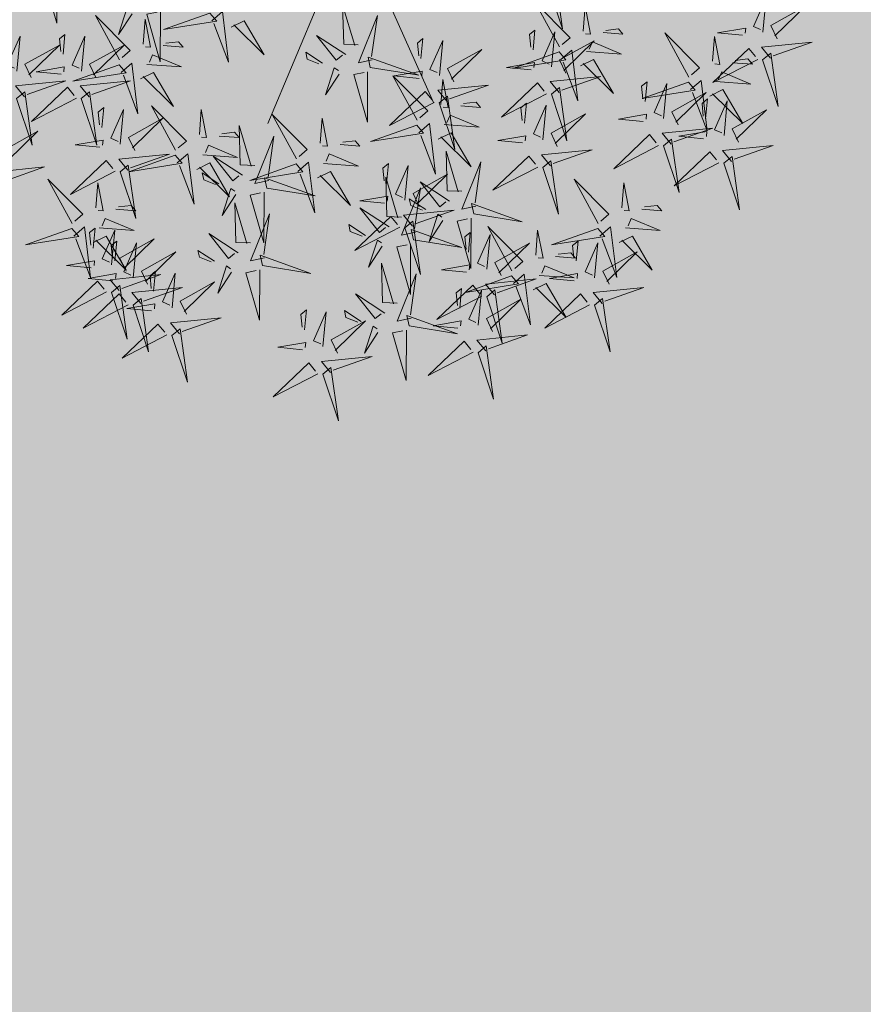
# Model space of a CAD drawing. Units: inches. Extents: x 1704 to 6393, y -157 to 1172.
# Tile 69 of 122: x 1928 to 1954, y 980 to 1010. Entities that reach past the tile are written whole.
import ezdxf

# ---------------------------------------------------------------- set-up
doc = ezdxf.new("R2010")
doc.units = ezdxf.units.IN
doc.header["$MEASUREMENT"] = 0
for name, color, linetype, lineweight in [('A-ANNO-DIMS', 7, 'Continuous', 13), ('L-shrub', 74, 'Continuous', 18), ('L-tree', 102, 'Continuous', 18)]:
    doc.layers.add(name, color=color, linetype=linetype, lineweight=lineweight)
doc.layers.add('L-HRDS-PATT', color=9, linetype='Continuous', lineweight=13, true_color=0xc5c1ba)
doc.styles.get("Standard").update_dxf_attribs({"font": 'arial.ttf'})
doc.dimstyles.get("Standard").update_dxf_attribs({"dimtxt": 6, "dimasz": 2, "dimexe": 0.18, "dimexo": 0.0625, "dimgap": 0.09, "dimtad": 0, "dimtih": 1, "dimtoh": 1, "dimdec": 1, "dimzin": 0, "dimdsep": 46, "dimlunit": 3, "dimtxsty": 'Standard', "dimblk": 'ARCHTICK', "dimcen": 0.09, "dimadec": 0, "dimazin": 0, "dimtfac": 1, "dimtdec": 1, "dimtofl": 0, "dimtmove": 0, "dimatfit": 3, "dimfxl": 1, "dimtolj": 1, "dimtzin": 0, "dimarcsym": 0})

# ---------------------------------------------------------------- blocks, each defined once
blk = doc.blocks.new('bamboo')
at = {"layer": 'L-shrub'}
for p, q in [((43.5, 73), (278.2, 631.2)), ((-12.4, 39.5), (-247.1, 564.2))]:
    blk.add_line(p, q, dxfattribs=at)
for points in [[(103.7, 1424.7), (54.4, 1572.3), (77.9, 1403.4), (103.7, 1424.7)], [(-387.8, 1356.5), (-437.1, 1504.1), (-413.6, 1335.2), (-387.8, 1356.5)], [(119.4, 1423.2), (261.4, 1496.7), (147.9, 1388.7), (126.6, 1414.5)], [(-160.7, 1284.9), (-160, 1444.8), (-116.9, 1294.1), (-149.7, 1287.2)], [(581.6, 1302), (532.2, 1449.6), (555.7, 1280.7), (581.6, 1302)], [(-372, 1355), (-230.1, 1428.5), (-343.6, 1320.5), (-364.9, 1346.4)], [(79.4, 1419.1), (107.8, 1384.6), (-52.4, 1368.4), (70.8, 1412)], [(597.3, 1300.4), (739.2, 1374), (625.7, 1265.9), (604.4, 1291.8)], [(-756.4, 1206.5), (-805.8, 1354.1), (-782.2, 1185.2), (-756.4, 1206.5)], [(-412.1, 1350.9), (-383.7, 1316.4), (-543.9, 1300.2), (-420.7, 1343.8)], [(-70.9, 1292.4), (-27.7, 1358.5), (-55.4, 1272.9), (-68.6, 1281.5)], [(57.7, 1357.7), (77.5, 1316.1), (-31.5, 1255.3), (64.8, 1349.1)], [(167.7, 1347.1), (246.3, 1339.5), (157.6, 1324.2), (159.1, 1340)], [(704.4, 1206.5), (655.1, 1354.1), (678.6, 1185.2), (704.4, 1206.5)], [(-415.1, 1179.2), (-464.4, 1326.8), (-440.9, 1157.9), (-415.1, 1179.2)], [(103.3, 1337.4), (92.8, 1227.4), (133.3, 1318.7), (110.4, 1328.8)], [(772.7, 1165.6), (723.3, 1313.2), (746.9, 1144.3), (772.7, 1165.6)], [(-740.7, 1205), (-598.8, 1278.5), (-712.2, 1170.5), (-733.6, 1196.4)], [(-433.8, 1289.5), (-414, 1248), (-523, 1187.1), (-426.7, 1280.9)], [(-323.8, 1278.9), (-245.2, 1271.3), (-333.9, 1256.1), (-332.4, 1271.8)], [(-169.3, 1271.7), (-323, 1296.4), (-162.4, 1238.9), (-169.3, 1271.7)], [(161.7, 1284.2), (155.7, 1221.3), (172.9, 1235.5), (168.8, 1275.6)], [(557.2, 1296.4), (585.7, 1261.9), (425.4, 1245.7), (548.6, 1289.3)], [(720.2, 1205), (862.1, 1278.5), (748.6, 1170.5), (727.3, 1196.4)], [(-500.1, 1137.3), (-534, 1108.2), (-553.5, 1268), (-507.4, 1145.8)], [(-399.4, 1177.7), (-257.4, 1251.3), (-370.9, 1143.2), (-392.2, 1169.1)], [(-388.2, 1269.3), (-398.7, 1159.2), (-358.2, 1250.5), (-381.1, 1260.6)], [(-175.7, 1247.6), (-131.9, 1256.8), (-191.9, 1107.3), (-173.4, 1236.6)], [(-92.2, 1230.9), (0.4, 1170.5), (-61.7, 1248.7), (-81.3, 1233.2)], [(-18, 1257.9), (35, 1223.4), (30.4, 1245.3), (-7, 1260.2)], [(303.5, 1094), (304.2, 1253.9), (347.3, 1103.2), (314.4, 1096.3)], [(-561.9, 1157.8), (-603.1, 1137.1), (-666.2, 1244.8), (-570.4, 1150.5)], [(-329.8, 1216), (-335.8, 1153.1), (-318.6, 1167.3), (-322.7, 1207.4)], [(535.5, 1235), (555.3, 1193.4), (446.4, 1132.5), (542.6, 1226.4)], [(645.6, 1224.3), (724.2, 1216.7), (635.4, 1201.5), (637, 1217.2)], [(788.4, 1164.1), (930.3, 1237.6), (816.9, 1129.6), (795.5, 1155.5)], [(-780.7, 1200.9), (-752.3, 1166.4), (-912.5, 1150.2), (-789.3, 1193.8)], [(-131.4, 1199.8), (-85.3, 1198.1), (-81.9, 1073.4), (-120.4, 1202.1)], [(680.1, 1200.9), (708.6, 1166.4), (548.3, 1150.2), (671.5, 1193.8)], [(581.2, 1214.7), (570.7, 1104.6), (611.1, 1195.9), (588.3, 1206.1)], [(-439.4, 1173.7), (-411, 1139.2), (-571.2, 1122.9), (-448, 1166.6)], [(-494, 1113.1), (-347.5, 1165.5), (-515.9, 1138.5), (-494, 1113.1)], [(-174.3, 1012.2), (-173.7, 1172.1), (-130.6, 1021.4), (-163.4, 1014.5)], [(393.3, 1101.5), (436.5, 1167.6), (408.8, 1082), (395.6, 1090.6)], [(748.4, 1160), (776.8, 1125.5), (616.6, 1109.3), (739.8, 1152.9)], [(639.6, 1161.5), (633.5, 1098.6), (650.8, 1112.8), (646.7, 1152.8)], [(-802.5, 1139.6), (-782.6, 1098), (-891.6, 1037.1), (-795.3, 1130.9)], [(-692.4, 1128.9), (-613.8, 1121.3), (-702.5, 1106.1), (-701, 1121.8)], [(658.4, 1139.6), (678.2, 1098), (569.2, 1037.1), (665.5, 1130.9)], [(768.4, 1128.9), (847.1, 1121.3), (758.3, 1106.1), (759.8, 1121.8)], [(-835, 1007.8), (-876.2, 987.1), (-939.2, 1094.8), (-843.4, 1000.5)], [(-773.2, 987.3), (-807.1, 958.2), (-826.6, 1118), (-780.4, 995.8)], [(-756.8, 1119.3), (-767.3, 1009.2), (-726.8, 1100.5), (-749.7, 1110.6)], [(-581.3, 1111.7), (-691.5, 1120), (-599.4, 1081.4), (-589.8, 1104.4)], [(-461.1, 1112.3), (-441.3, 1070.7), (-550.3, 1009.8), (-454, 1103.7)], [(-495.2, 1097.3), (-418.8, 957), (-529.1, 1068.2), (-503.7, 1090.1)], [(-415.5, 1092), (-426, 981.9), (-385.5, 1073.2), (-408.4, 1083.4)], [(-351.1, 1101.6), (-272.5, 1094), (-361.2, 1078.8), (-359.7, 1094.5)], [(-155.7, 961.1), (-205, 1108.7), (-181.5, 939.8), (-155.7, 961.1)], [(294.9, 1080.8), (141.2, 1105.5), (301.8, 1048), (294.9, 1080.8)], [(726.6, 1098.6), (746.5, 1057), (637.5, 996.2), (733.8, 1090)], [(704, 1119.3), (693.5, 1009.2), (734, 1100.5), (711.2, 1110.6)], [(830.7, 1007.8), (789.5, 987.1), (726.4, 1094.8), (822.2, 1000.5)], [(892.5, 987.3), (858.6, 958.2), (839.1, 1118), (885.2, 995.8)], [(-698.4, 1066), (-704.4, 1003.1), (-687.2, 1017.3), (-691.3, 1057.4)], [(-365.5, 930.4), (-364.8, 1090.2), (-321.7, 939.6), (-354.5, 932.7)], [(-84.5, 1019.7), (-41.3, 1085.8), (-69, 1000.1), (-82.2, 1008.8)], [(288.5, 1056.7), (332.3, 1065.9), (272.3, 916.4), (290.8, 1045.7)], [(446.2, 1067), (499.2, 1032.5), (494.6, 1054.4), (457.2, 1069.3)], [(762.4, 1066), (756.4, 1003.1), (773.6, 1017.3), (769.5, 1057.4)], [(772.3, 1078.4), (761.8, 968.3), (802.3, 1059.6), (779.4, 1069.7)], [(836.7, 1088), (915.3, 1080.4), (826.6, 1065.2), (828.1, 1080.9)], [(-633.3, 1052.3), (-696.3, 1057), (-681.8, 1040.1), (-641.8, 1045)], [(-570.3, 1047.5), (-576.3, 968.8), (-593.4, 1057.2), (-577.6, 1056)], [(-357.1, 1038.7), (-363.1, 975.8), (-345.9, 990), (-350, 1030.1)], [(-140, 959.5), (2, 1033.1), (-111.5, 925), (-132.8, 950.9)], [(372, 1040), (464.6, 979.6), (402.5, 1057.8), (382.9, 1042.3)], [(-767.1, 963.1), (-620.5, 1015.5), (-788.9, 988.5), (-767.1, 963.1)], [(-183, 999), (-336.7, 1023.7), (-176.1, 966.2), (-183, 999)], [(-275.7, 937.9), (-232.5, 1004), (-260.1, 918.3), (-273.4, 927)], [(289.9, 848.6), (290.5, 1008.4), (333.6, 857.8), (300.8, 850.9)], [(332.8, 1008.9), (378.9, 1007.2), (382.3, 882.5), (343.8, 1011.2)], [(830.7, 1025.1), (824.7, 962.2), (841.9, 976.4), (837.8, 1016.5)], [(898.5, 963.1), (1045.1, 1015.5), (876.7, 988.5), (898.5, 963.1)], [(-854.3, 961.7), (-964.6, 970), (-872.5, 931.4), (-862.8, 954.4)], [(-189.3, 974.8), (-145.6, 984), (-205.5, 834.6), (-187, 963.9)], [(-105.9, 958.2), (-13.2, 897.8), (-75.4, 976), (-94.9, 960.5)], [(-31.6, 985.2), (21.3, 950.7), (16.7, 972.5), (-20.7, 987.5)], [(811.3, 961.7), (701, 970), (793.1, 931.4), (802.8, 954.4)], [(-768.3, 947.3), (-691.9, 807), (-802.2, 918.2), (-776.8, 940.1)], [(-374.1, 917.2), (-527.8, 941.9), (-367.2, 884.4), (-374.1, 917.2)], [(-180, 955.5), (-151.6, 921), (-311.8, 904.8), (-188.6, 948.4)], [(897.3, 947.3), (973.8, 807), (863.4, 918.2), (888.9, 940.1)], [(-1166, 756.5), (-1215.3, 904.1), (-1191.8, 735.2), (-1166, 756.5)], [(-906.4, 902.3), (-969.4, 907), (-954.8, 890.1), (-914.9, 895)], [(-843.4, 897.5), (-849.4, 818.8), (-866.4, 907.2), (-850.7, 906)], [(-592.6, 770.2), (-641.9, 917.8), (-618.4, 748.9), (-592.6, 770.2)], [(-222.7, 903.4), (-169.8, 868.9), (-174.4, 890.7), (-211.8, 905.7)], [(-145, 927.1), (-99, 925.4), (-95.6, 800.6), (-134.1, 929.4)], [(182.5, 782.8), (148.6, 753.6), (129.1, 913.5), (175.2, 791.2)], [(379.6, 856.1), (422.9, 922.2), (395.2, 836.5), (381.9, 845.1)], [(745.4, 783.8), (696, 931.4), (719.6, 762.5), (745.4, 783.8)], [(759.2, 902.3), (696.2, 907), (710.8, 890.1), (750.8, 895)], [(822.2, 897.5), (816.2, 818.8), (799.2, 907.2), (815, 906)], [(-380.5, 893), (-336.7, 902.2), (-396.6, 752.7), (-378.2, 882.1)], [(-297, 876.4), (-204.4, 816), (-266.5, 894.2), (-286.1, 878.7)], [(-201.7, 894.1), (-181.9, 852.5), (-290.9, 791.6), (-194.6, 885.5)], [(-156.1, 873.8), (-166.6, 763.7), (-126.1, 855), (-149, 865.2)], [(-91.7, 883.5), (-13.1, 875.8), (-101.8, 860.6), (-100.3, 876.4)], [(120.7, 803.3), (79.5, 782.6), (16.5, 890.3), (112.2, 796)], [(564.8, 755.5), (530.9, 726.4), (511.4, 886.2), (557.5, 764)], [(-974.8, 702), (-1024.2, 849.6), (-1000.7, 680.7), (-974.8, 702)], [(-576.8, 768.6), (-434.9, 842.2), (-548.4, 734.1), (-569.7, 760)], [(-336.2, 845.3), (-290.1, 843.6), (-286.7, 718.8), (-325.2, 847.6)], [(281.2, 835.4), (127.5, 860.1), (288.1, 802.6), (281.2, 835.4)], [(503, 776), (461.8, 755.3), (398.7, 863), (494.5, 768.7)], [(761.1, 782.3), (903, 855.8), (789.6, 747.8), (768.2, 773.7)], [(-1150.2, 755), (-1008.3, 828.6), (-1121.8, 720.5), (-1143.1, 746.4)], [(-97.7, 820.6), (-103.7, 757.7), (-86.5, 771.9), (-90.6, 811.9)], [(188.6, 758.6), (335.2, 810.9), (166.8, 784), (188.6, 758.6)], [(274.9, 811.2), (318.6, 820.4), (258.7, 670.9), (277.2, 800.3)], [(358.3, 794.5), (451, 734.2), (388.8, 812.4), (369.3, 796.8)], [(432.6, 821.6), (485.5, 787.1), (480.9, 808.9), (443.5, 823.9)], [(1117, 819.1), (1145.4, 784.6), (985.2, 768.4), (1108.4, 812)], [(-199.8, 660.1), (-233.7, 630.9), (-253.2, 790.8), (-207, 668.5)], [(570.9, 731.3), (717.4, 783.7), (549, 756.7), (570.9, 731.3)], [(-1190.3, 750.9), (-1161.9, 716.5), (-1322.1, 700.2), (-1198.9, 743.8)], [(-959.1, 700.5), (-817.2, 774), (-930.7, 666), (-952, 691.8)], [(-616.9, 764.6), (-588.5, 730.1), (-748.7, 713.9), (-625.5, 757.5)], [(-261.6, 680.5), (-302.7, 659.9), (-365.8, 767.6), (-270, 673.2)], [(101.4, 757.2), (-8.9, 765.5), (83.2, 726.9), (92.9, 749.9)], [(319.2, 763.5), (365.2, 761.8), (368.6, 637), (330.1, 765.8)], [(721.1, 778.2), (749.5, 743.7), (589.3, 727.5), (712.5, 771.1)], [(1095.3, 757.7), (1115.1, 716.2), (1006.1, 655.3), (1102.4, 749.1)], [(187.4, 742.8), (263.8, 602.4), (153.5, 713.7), (178.9, 735.5)], [(483.6, 729.9), (373.4, 738.2), (465.5, 699.6), (475.2, 722.6)], [(-1212, 689.6), (-1192.2, 648), (-1301.2, 587.1), (-1204.9, 680.9)], [(-999.2, 696.4), (-970.7, 661.9), (-1131, 645.7), (-1007.8, 689.3)], [(-638.6, 703.2), (-618.8, 661.6), (-727.8, 600.7), (-631.5, 694.6)], [(-619.9, 538.4), (-669.2, 686), (-645.7, 517), (-619.9, 538.4)], [(-528.6, 692.6), (-450, 684.9), (-538.7, 669.7), (-537.2, 685.5)], [(-264.9, 565.6), (-314.3, 713.2), (-290.7, 544.3), (-264.9, 565.6)], [(-193.7, 635.8), (-47.1, 688.2), (-215.5, 661.2), (-193.7, 635.8)], [(49.3, 697.7), (-13.7, 702.5), (0.8, 685.5), (40.8, 690.4)], [(112.3, 693), (106.3, 614.2), (89.3, 702.6), (105, 701.5)], [(569.7, 715.5), (646.1, 575.2), (535.8, 686.4), (561.2, 708.3)], [(699.3, 716.8), (719.2, 675.2), (610.2, 614.4), (706.4, 708.2)], [(745, 696.6), (734.5, 586.5), (774.9, 677.8), (752.1, 687.9)], [(809.4, 706.2), (888, 698.6), (799.3, 683.4), (800.8, 699.1)], [(868.3, 552), (818.9, 699.6), (842.4, 530.7), (868.3, 552)], [(1073.1, 552), (1023.7, 699.6), (1047.2, 530.7), (1073.1, 552)], [(-1166.4, 669.3), (-1176.9, 559.2), (-1136.4, 650.5), (-1159.3, 660.7)], [(-1102, 678.9), (-1023.4, 671.3), (-1112.1, 656.1), (-1110.6, 671.8)], [(-593, 682.9), (-603.5, 572.8), (-563, 664.1), (-585.9, 674.3)], [(431.6, 670.5), (368.6, 675.2), (383.1, 658.2), (423.1, 663.2)], [(494.6, 665.7), (488.6, 587), (471.6, 675.4), (487.3, 674.2)], [(-1121.7, 544.2), (-1162.9, 523.5), (-1225.9, 631.2), (-1130.2, 536.9)], [(-1059.9, 523.7), (-1093.8, 494.6), (-1113.3, 654.4), (-1067.1, 532.2)], [(-1020.9, 635), (-1001.1, 593.4), (-1110, 532.6), (-1013.8, 626.4)], [(-910.8, 624.4), (-832.2, 616.8), (-921, 601.5), (-919.5, 617.3)], [(-534.6, 629.7), (-540.6, 566.8), (-523.4, 581), (-527.5, 621)], [(-280.9, 634.5), (-391.2, 642.7), (-299.1, 604.1), (-289.4, 627.2)], [(-249.2, 564.1), (-107.3, 637.7), (-220.7, 529.6), (-242.1, 555.5)], [(-37.8, 466.8), (-37.2, 626.6), (5.9, 476), (-26.9, 469.1)], [(803.4, 643.3), (797.4, 580.4), (814.6, 594.6), (810.5, 634.7)], [(884, 550.5), (1025.9, 624), (912.4, 516), (891.1, 541.8)], [(-1108, 616), (-1114, 553.1), (-1096.8, 567.3), (-1100.9, 607.4)], [(-975.2, 614.7), (-985.8, 504.7), (-945.3, 596), (-968.1, 606.1)], [(-604.1, 536.8), (-462.2, 610.4), (-575.7, 502.3), (-597, 528.2)], [(-194.9, 620.1), (-118.4, 479.7), (-228.8, 591), (-203.4, 612.8)], [(742.3, 469.2), (708.4, 440), (688.9, 599.9), (735, 477.6)], [(-1288.8, 429.3), (-1338.2, 576.9), (-1314.7, 408), (-1288.8, 429.3)], [(-916.9, 561.5), (-922.9, 498.6), (-905.6, 512.8), (-909.7, 552.9)], [(-333, 575), (-396, 579.7), (-381.4, 562.8), (-341.5, 567.7)], [(-270, 570.3), (-276, 491.5), (-293, 579.9), (-277.2, 578.7)], [(680.5, 489.6), (639.3, 469), (576.2, 576.7), (672, 482.3)], [(-1053.8, 499.5), (-907.2, 551.9), (-1075.6, 524.9), (-1053.8, 499.5)], [(-712.1, 448.7), (-753.3, 428.1), (-816.4, 535.7), (-720.6, 441.4)], [(-644.2, 532.8), (-615.8, 498.3), (-776, 482), (-652.8, 525.7)], [(-650.3, 428.2), (-684.2, 399.1), (-703.7, 559), (-657.6, 436.7)], [(-289.2, 560), (-260.8, 525.6), (-421, 509.3), (-297.8, 552.9)], [(52, 474.3), (95.2, 540.4), (67.5, 454.7), (54.3, 463.3)], [(843.9, 546.4), (872.4, 511.9), (712.1, 495.7), (835.3, 539.3)], [(1048.7, 546.4), (1077.2, 511.9), (916.9, 495.7), (1040.1, 539.3)], [(-1273.1, 427.7), (-1131.2, 501.3), (-1244.7, 393.3), (-1266, 419.1)], [(-1141, 498.1), (-1251.3, 506.4), (-1159.2, 467.8), (-1149.5, 490.8)], [(-1055, 483.7), (-978.6, 343.4), (-1088.9, 454.6), (-1063.5, 476.4)], [(-665.9, 471.4), (-646.1, 429.8), (-755.1, 368.9), (-658.8, 462.8)], [(-311, 498.7), (-291.1, 457.1), (-400.1, 396.2), (-303.9, 490)], [(-265.3, 478.4), (-275.8, 368.3), (-235.4, 459.6), (-258.2, 469.8)], [(-200.9, 488), (-122.3, 480.4), (-211, 465.2), (-209.5, 480.9)], [(-46.5, 453.6), (-200.1, 478.3), (-39.6, 420.8), (-46.5, 453.6)], [(748.4, 444.9), (894.9, 497.3), (726.5, 470.3), (748.4, 444.9)], [(822.2, 485), (842, 443.4), (733.1, 382.6), (829.3, 476.4)], [(932.3, 474.4), (1010.9, 466.8), (922.2, 451.6), (923.7, 467.3)], [(1027, 485), (1046.8, 443.4), (937.9, 382.6), (1034.1, 476.4)], [(-1193.1, 438.6), (-1256.1, 443.4), (-1241.5, 426.4), (-1201.6, 431.4)], [(-1130.1, 433.9), (-1136.1, 355.2), (-1153.1, 443.6), (-1137.4, 442.4)], [(-644.2, 404), (-497.6, 456.4), (-666, 429.4), (-644.2, 404)], [(-620.3, 451.1), (-630.8, 341), (-590.3, 432.3), (-613.2, 442.5)], [(-555.9, 460.7), (-477.3, 453.1), (-566, 437.9), (-564.5, 453.6)], [(-52.8, 429.4), (-9, 438.6), (-69, 289.1), (-50.5, 418.5)], [(104.9, 439.8), (157.9, 405.3), (153.3, 427.1), (115.9, 442.1)], [(661.1, 443.6), (550.9, 451.8), (643, 413.2), (652.6, 436.3)], [(867.9, 464.7), (857.4, 354.7), (897.8, 446), (875, 456.1)], [(1072.7, 464.7), (1062.1, 354.7), (1102.6, 446), (1079.8, 456.1)], [(-1313.2, 423.7), (-1284.7, 389.2), (-1445, 373), (-1321.8, 416.6)], [(-731.5, 402.7), (-841.7, 410.9), (-749.6, 372.3), (-739.9, 395.4)], [(-206.9, 425.1), (-212.9, 362.2), (-195.7, 376.4), (-199.8, 416.5)], [(30.7, 412.7), (123.3, 352.4), (61.2, 430.6), (41.6, 415)], [(393.8, 326), (352.6, 305.3), (289.5, 413), (385.3, 318.7)], [(455.6, 305.5), (421.7, 276.4), (402.2, 436.3), (448.3, 314)], [(617.5, 275.9), (618.2, 435.7), (661.3, 285.1), (628.5, 278.2)], [(747.2, 429.2), (823.6, 288.8), (713.3, 400), (738.7, 421.9)], [(926.3, 411.5), (920.3, 348.6), (937.5, 362.8), (933.4, 402.9)], [(-645.4, 388.3), (-569, 247.9), (-679.3, 359.1), (-653.9, 381)], [(-561.9, 397.8), (-567.9, 334.9), (-550.7, 349.1), (-554.8, 389.2)], [(-8.5, 381.7), (37.5, 380), (40.9, 255.2), (2.4, 384)], [(609.1, 384.1), (546.1, 388.8), (560.6, 371.9), (600.6, 376.8)], [(672.1, 379.4), (666.1, 300.6), (649, 389), (664.8, 387.8)], [(-1334.9, 362.3), (-1315.1, 320.7), (-1424, 259.8), (-1327.8, 353.7)], [(-1224.9, 351.7), (-1146.2, 344), (-1235, 328.8), (-1233.5, 344.6)], [(-783.5, 343.2), (-846.5, 347.9), (-832, 331), (-792, 335.9)], [(-720.5, 338.5), (-726.5, 259.7), (-743.5, 348.1), (-727.8, 346.9)], [(707.3, 283.4), (750.5, 349.5), (722.8, 263.8), (709.6, 272.4)], [(-1289.2, 342), (-1299.8, 231.9), (-1259.3, 323.3), (-1282.1, 333.4)], [(-606.2, 183.8), (-655.6, 331.4), (-632, 162.5), (-606.2, 183.8)], [(461.7, 281.3), (608.2, 333.7), (439.8, 306.7), (461.7, 281.3)], [(945.2, 153.2), (945.8, 313), (988.9, 162.4), (956.1, 155.5)]]:
    blk.add_lwpolyline(points, dxfattribs=at)
blk = doc.blocks.new('_ArchTick')
at = {"color": 0, "linetype": 'ByBlock', "const_width": 0.15}
blk.add_lwpolyline([(-0.5, -0.5), (0.5, 0.5)], dxfattribs=at)
blk = doc.blocks.new('*D94')
at = {"layer": 'A-ANNO-DIMS', "color": 0, "lineweight": -2, "transparency": 16777216}
for p, q in [((1898.349, 895.275), (1898.349, 1105.287)), ((2073.349, 895.275), (2073.349, 1105.287)), ((1898.349, 1105.107), (1979.39, 1105.107)), ((2073.349, 1105.107), (1992.307, 1105.107))]:
    blk.add_line(p, q, dxfattribs=at)
at = {"layer": 'Defpoints', "color": 0, "lineweight": -3, "transparency": 16777216}
for p in [(2073.349, 1105.107), (1898.349, 895.213), (2073.349, 895.213)]:
    blk.add_point(p, dxfattribs=at)
at = {"layer": 'A-ANNO-DIMS', "color": 0, "lineweight": -2, "transparency": 16777216, "xscale": 2, "yscale": 2, "zscale": 2, "rotation": 180}
blk.add_blockref('_ArchTick', (1898.349, 1105.107), dxfattribs=at)
at = {"layer": 'A-ANNO-DIMS', "color": 0, "lineweight": -2, "transparency": 16777216, "xscale": 2, "yscale": 2, "zscale": 2}
blk.add_blockref('_ArchTick', (2073.349, 1105.107), dxfattribs=at)
at = {"layer": 'A-ANNO-DIMS', "color": 0, "transparency": 16777216, "insert": (1985.849, 1105.107), "char_height": 6, "attachment_point": 5}
blk.add_mtext('\\A1;175', dxfattribs=at)

msp = doc.modelspace()

# ---------------------------------------------------------------- hatches: boundary and pattern name
at = {"layer": 'L-HRDS-PATT', "transparency": 33554643}
h = msp.add_hatch(color=256, dxfattribs=at)
h.dxf.hatch_style = 1
h.paths.add_polyline_path([(2065.589, 1033.213), (1898.349, 1033.213), (1898.349, 895.213), (2065.589, 895.213)])

# ---------------------------------------------------------------- block references
at = {"layer": 'L-tree', "xscale": 0.0095734028514679, "yscale": 0.0095734028514679, "zscale": 0.0095734028514679, "rotation": 180}
msp.add_blockref('bamboo', (1938.628, 1012.792), dxfattribs=at)

# ---------------------------------------------------------------- dimensions: what is measured, and where the dimension line sits
at = {"layer": 'A-ANNO-DIMS'}
dim = msp.add_linear_dim(base=(2073.349, 1105.107), p1=(1898.349, 895.213), p2=(2073.349, 895.213), dimstyle='Standard', override={"dimdec": 0, "dimlfac": 1, "dimrnd": 0, "dimzin": 0, "dimdsep": 46, "dimlunit": 2}, dxfattribs=at)
dim.commit()
dim.dimension.update_dxf_attribs({"geometry": '*D94', "text_midpoint": (1985.849, 1105.107)})

doc.saveas('drawing.dxf')
